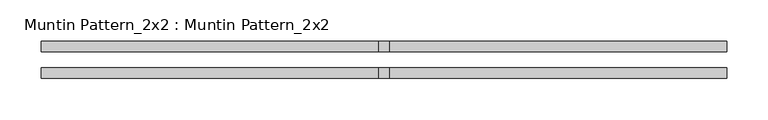
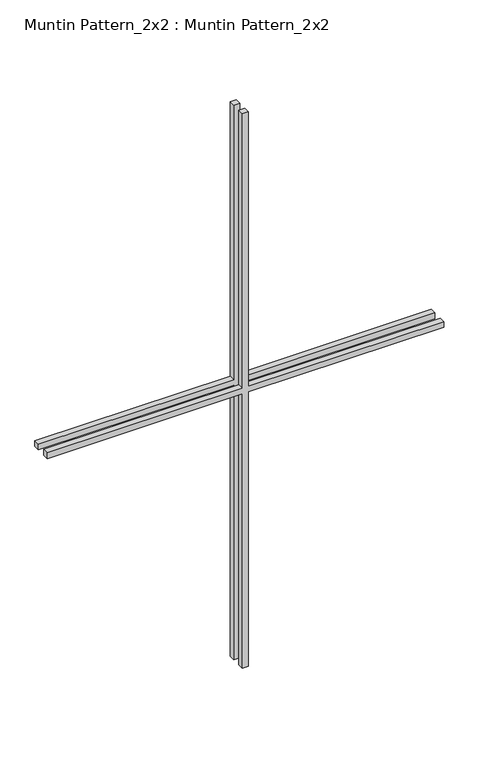
"""IFC4 building model written with IfcOpenShell, lengths in millimetres: proxy geometry, Muntin Pattern_2x2 : Muntin Pattern_2x2."""

from ifc_helpers import new_model, si_unit, frame, origin, place, context, project, spatial, polyline, outline, extrude, source, transform, mapped, element, save


def muntin_pattern_2x2_muntin_pattern_2x2_4a783bbe(model_context):
    return source(origin(), model_context, "Body", "SweptSolid", [
        extrude(outline(polyline([(619.125, -6.35), (619.125, -414.3375), (606.425, -414.3375), (606.425, -6.35), (0.0, -6.35), (0.0, 6.35), (606.425, 6.35), (606.425, 414.3375), (619.125, 414.3375), (619.125, 6.35), (1225.55, 6.35), (1225.55, -6.35), (619.125, -6.35)])), frame((0.0, 9.525, 0.0), z_axis=(0.0, 1.0, 0.0), x_axis=(0.0, 0.0, 1.0)), (0.0, 0.0, 1.0), 12.7),
        extrude(outline(polyline([(619.125, -6.35), (619.125, -414.3375), (606.425, -414.3375), (606.425, -6.35), (0.0, -6.35), (0.0, 6.35), (606.425, 6.35), (606.425, 414.3375), (619.125, 414.3375), (619.125, 6.35), (1225.55, 6.35), (1225.55, -6.35), (619.125, -6.35)])), frame((0.0, -22.225, 0.0), z_axis=(0.0, 1.0, 0.0), x_axis=(0.0, 0.0, 1.0)), (0.0, 0.0, 1.0), 12.7),
    ])


if __name__ == "__main__":
    model = new_model("IFC4")
    model_context = context("Model", 3, world=origin())
    ifc_project = project(units=[si_unit("LENGTHUNIT", "METRE", prefix="MILLI")], contexts=[model_context])
    site = spatial("IfcSite", under=ifc_project)
    building = spatial("IfcBuilding", under=site)
    placement = place(None, origin())
    muntin_pattern_2x2_muntin_pattern_2x2_shape = muntin_pattern_2x2_muntin_pattern_2x2_4a783bbe(model_context)
    element("IfcBuildingElementProxy", 1, Name="Muntin Pattern_2x2 : Muntin Pattern_2x2", ObjectType="Muntin Pattern_2x2 : Muntin Pattern_2x2", at=placement, inside=building, context=model_context, shape_type="MappedRepresentation", body=[
        mapped(muntin_pattern_2x2_muntin_pattern_2x2_shape, transform((0.0, 0.0, 0.0), x_axis=(1.0, 0.0, 0.0), y_axis=(0.0, 1.0, 0.0), z_axis=(0.0, 0.0, 1.0))),
    ])
    save(model, "model.ifc")

# Revit data of these elements
# Type "Muntin Pattern_2x2 : Muntin Pattern_2x2"
#   Width [instance default] = 4' - 0"
#   Thickness = 0' - 0 1/2"
#   Height [instance default] = 4' - 0"
#   Distance = 0' - 0 3/4"
#   Interior Material [instance default] = none
#   Exterior Material [instance default] = none
#   Default Elevation = 0
# Element 1 (IfcBuildingElementProxy, "Muntin Pattern_2x2 : Muntin Pattern_2x2")
#   Width = 2' - 8 5/8"
#   Height = 4' - 0 1/4"
#   Interior Material = Wood - Stained
#   Exterior Material = Clad - White
#   Materials on its faces: "Clad - White", "Wood - Stained"
# Materials
#   "Clad - White": class "Wood", colour RGB 242 242 238, transparency 0, Cost = 0
#   "Wood - Stained": class "Wood", colour RGB 224 178 126, transparency 0, Cost = 0
